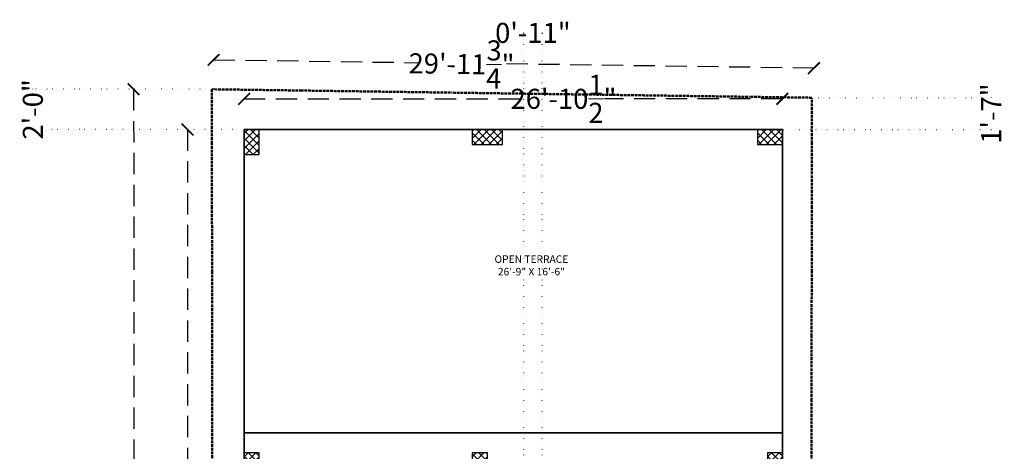
# Model space of a CAD drawing. Units: inches. Extents: x -16911 to -9621, y -48626 to -46270.
# Tile 19 of 20: x -11596 to -11006, y -46579 to -46321. Entities that reach past the tile are written whole.
import ezdxf

# ---------------------------------------------------------------- set-up
doc = ezdxf.new("R2010")
doc.units = ezdxf.units.IN
for name, pattern in [('DASHDOT', [1, 0.5, -0.25, 0, -0.25]), ('DASHED', [19.05, 12.7, -6.35]), ('DOT2', [3.175, 0, -3.175])]:
    doc.linetypes.add(name, pattern=pattern)
for name, color, linetype, lineweight in [('A-ANNO-DIMS', 2, 'Continuous', 13), ('A-AREA-IDEN', 3, 'Continuous', 18), ('A-WALL', 7, 'Continuous', 35), ('C-PROP', 6, 'DASHDOT', 50), ('column', 12, 'Continuous', 30), ('S-COLS', 1, 'Continuous', 30)]:
    doc.layers.add(name, color=color, linetype=linetype, lineweight=lineweight)
doc.styles.add('style9', font='swisscl.ttf', dxfattribs={"height": 12})
doc.dimstyles.new('Dim9', dxfattribs={"dimtxt": 10, "dimasz": 0.199219, "dimexe": 1, "dimexo": 0.5, "dimgap": 1, "dimtad": 0, "dimdec": 1, "dimzin": 0, "dimdsep": 46, "dimlunit": 4, "dimtxsty": 'style9', "dimblk": 'ARCHTICK', "dimcen": 0.09, "dimclrd": 256, "dimclrt": 256, "dimadec": 0, "dimazin": 0, "dimtfac": 1, "dimtdec": 1, "dimtix": 1, "dimtofl": 0, "dimtmove": 1, "dimatfit": 3, "dimfxl": 9, "dimtolj": 1, "dimtzin": 0, "dimlwd": -1, "dimarcsym": 0})

# ---------------------------------------------------------------- blocks, each defined once
blk = doc.blocks.new('_ArchTick')
at = {"color": 0, "linetype": 'ByBlock', "const_width": 0.15}
blk.add_lwpolyline([(-0.5, -0.5), (0.5, 0.5)], dxfattribs=at)
blk = doc.blocks.new('*D12')
at = {"layer": 'A-ANNO-DIMS', "color": 0, "linetype": 'DOT2', "lineweight": -2, "transparency": 16777216}
for p, q in [((-11479.71, -46345.34), (-11479.69, -46344.15)), ((-11120.05, -46350.39), (-11120.03, -46349.2))]:
    blk.add_line(p, q, dxfattribs=at)
at = {"layer": 'A-ANNO-DIMS', "color": 0, "linetype": 'DASHED', "lineweight": 25, "transparency": 16777216}
for p, q in [((-11479.71, -46345.15), (-11355.97, -46346.89)), ((-11120.04, -46350.2), (-11306.38, -46347.59))]:
    blk.add_line(p, q, dxfattribs=at)
at = {"layer": 'Defpoints', "color": 0, "transparency": 16777216}
for p in [(-11120.04, -46350.2), (-11479.9, -46359.07), (-11120.24, -46364.11)]:
    blk.add_point(p, dxfattribs=at)
at = {"layer": 'A-ANNO-DIMS', "color": 0, "lineweight": 25, "transparency": 16777216, "xscale": 7, "yscale": 7, "zscale": 7}
for p, rotation in [((-11479.71, -46345.15), 179.1963905603631), ((-11120.04, -46350.2), 359.196390560363)]:
    blk.add_blockref('_ArchTick', p, dxfattribs=dict(at, rotation=rotation))
at = {"layer": 'A-ANNO-DIMS', "color": 0, "transparency": 16777216, "insert": (-11331.18, -46347.68), "char_height": 12, "attachment_point": 5, "rotation": 359.19639, "style": 'style9'}
blk.add_mtext('\\A1;29\'-11{\\H1x;\\S3/4;}"', dxfattribs=at)
blk = doc.blocks.new('*D13')
at = {"layer": 'A-ANNO-DIMS', "color": 0, "linetype": 'DOT2', "lineweight": -2, "transparency": 16777216}
for p, q in [((-11527.5, -46362.82), (-11528.69, -46362.82)), ((-11527.14, -46962.82), (-11528.32, -46962.82))]:
    blk.add_line(p, q, dxfattribs=at)
at = {"layer": 'A-ANNO-DIMS', "color": 0, "linetype": 'DASHED', "lineweight": 25, "transparency": 16777216}
for p, q in [((-11527.69, -46362.82), (-11527.51, -46653.98)), ((-11527.32, -46962.82), (-11527.5, -46671.67))]:
    blk.add_line(p, q, dxfattribs=at)
at = {"layer": 'Defpoints', "color": 0, "transparency": 16777216}
for p in [(-11527.69, -46362.82), (-11508.87, -46362.81), (-11508.51, -46962.81)]:
    blk.add_point(p, dxfattribs=at)
at = {"layer": 'A-ANNO-DIMS', "color": 0, "lineweight": 25, "transparency": 16777216, "xscale": 7, "yscale": 7, "zscale": 7}
for p, rotation in [((-11527.69, -46362.82), 90.0346840750536), ((-11527.32, -46962.82), 270.0346840750536)]:
    blk.add_blockref('_ArchTick', p, dxfattribs=dict(at, rotation=rotation))
at = {"layer": 'A-ANNO-DIMS', "color": 0, "transparency": 16777216, "insert": (-11527.51, -46662.82), "char_height": 12, "attachment_point": 5, "rotation": 270.03468, "style": 'style9'}
blk.add_mtext("\\A1;50'", dxfattribs=at)
blk = doc.blocks.new('*D14')
at = {"layer": 'A-ANNO-DIMS', "color": 0, "linetype": 'DOT2', "lineweight": -2, "transparency": 16777216}
for p, q in [((-11461.47, -46368.33), (-11461.47, -46369.52)), ((-11138.92, -46368.33), (-11138.92, -46369.52))]:
    blk.add_line(p, q, dxfattribs=at)
at = {"layer": 'A-ANNO-DIMS', "color": 0, "linetype": 'DASHED', "lineweight": 25, "transparency": 16777216}
for p, q in [((-11461.47, -46368.52), (-11294.69, -46368.52)), ((-11138.92, -46368.52), (-11245.42, -46368.52))]:
    blk.add_line(p, q, dxfattribs=at)
at = {"layer": 'Defpoints', "color": 0, "transparency": 16777216}
for p in [(-11461.47, -46345.28), (-11138.92, -46345.28), (-11138.92, -46368.52)]:
    blk.add_point(p, dxfattribs=at)
at = {"layer": 'A-ANNO-DIMS', "color": 0, "lineweight": 25, "transparency": 16777216, "xscale": 7, "yscale": 7, "zscale": 7, "rotation": 180}
blk.add_blockref('_ArchTick', (-11461.47, -46368.52), dxfattribs=at)
at = {"layer": 'A-ANNO-DIMS', "color": 0, "lineweight": 25, "transparency": 16777216, "xscale": 7, "yscale": 7, "zscale": 7}
blk.add_blockref('_ArchTick', (-11138.92, -46368.52), dxfattribs=at)
at = {"layer": 'A-ANNO-DIMS', "color": 0, "transparency": 16777216, "insert": (-11270.06, -46368.52), "char_height": 12, "attachment_point": 5, "style": 'style9'}
blk.add_mtext('\\A1;26\'-10{\\H1x;\\S1/2;}"', dxfattribs=at)
blk = doc.blocks.new('*D15')
at = {"layer": 'A-ANNO-DIMS', "color": 0, "linetype": 'DOT2', "lineweight": -2, "transparency": 16777216}
for p, q in [((-11495.22, -46386.86), (-11496.4, -46386.86)), ((-11495.22, -46944.81), (-11496.4, -46944.81))]:
    blk.add_line(p, q, dxfattribs=at)
at = {"layer": 'A-ANNO-DIMS', "color": 0, "linetype": 'DASHED', "lineweight": 25, "transparency": 16777216}
for p, q in [((-11495.4, -46386.86), (-11495.4, -46648.2)), ((-11495.4, -46944.81), (-11495.4, -46683.47))]:
    blk.add_line(p, q, dxfattribs=at)
at = {"layer": 'Defpoints', "color": 0, "transparency": 16777216}
for p in [(-11461.47, -46386.86), (-11495.4, -46944.81), (-11461.47, -46944.81)]:
    blk.add_point(p, dxfattribs=at)
at = {"layer": 'A-ANNO-DIMS', "color": 0, "lineweight": 25, "transparency": 16777216, "xscale": 7, "yscale": 7, "zscale": 7}
for p, rotation in [((-11495.4, -46386.86), 90), ((-11495.4, -46944.81), 270)]:
    blk.add_blockref('_ArchTick', p, dxfattribs=dict(at, rotation=rotation))
at = {"layer": 'A-ANNO-DIMS', "color": 0, "transparency": 16777216, "insert": (-11495.4, -46665.83), "char_height": 12, "attachment_point": 5, "rotation": 90, "style": 'style9'}
blk.add_mtext('\\A1;46\'-6"', dxfattribs=at)
blk = doc.blocks.new('COLUMNS')
at = {"layer": 'column'}
h = blk.add_hatch(dxfattribs=at)
h.set_pattern_fill('ANSI37', color=256, angle=-720)
h.set_pattern_definition([(45, (21703.4588, -104481.6704), (-2.24506403, 2.24506403), []), (135, (21703.4588, -104481.6704), (-2.24506403, -2.24506403), [])])
h.paths.add_polyline_path([(-12061.47, -46401.86), (-12052.47, -46401.86), (-12052.47, -46386.86), (-12061.47, -46386.86)])
h = blk.add_hatch(dxfattribs=at)
h.set_pattern_fill('ANSI37', color=256, angle=-810)
h.set_pattern_definition([(315, (-70004.5392, -80151.7886), (2.24506403, 2.24506403), []), (45, (-70004.5392, -80151.7886), (-2.24506403, 2.24506403), [])])
h.paths.add_polyline_path([(-11924.72, -46386.86), (-11924.72, -46395.86), (-11906.72, -46395.86), (-11906.72, -46386.86)])
h = blk.add_hatch(dxfattribs=at)
h.set_pattern_fill('ANSI37', color=256, angle=-810)
h.set_pattern_definition([(315, (-69833.7395, -80151.7886), (2.24506403, 2.24506403), []), (45, (-69833.7395, -80151.7886), (-2.24506403, 2.24506403), [])])
h.paths.add_polyline_path([(-11753.92, -46386.86), (-11753.92, -46395.86), (-11738.92, -46395.86), (-11738.92, -46386.86)])
h = blk.add_hatch(dxfattribs=at)
h.set_pattern_fill('ANSI37', color=256, angle=-900)
h.set_pattern_definition([(225, (-45817.4075, 11499.4594), (2.24506403, -2.24506403), []), (315, (-45817.4075, 11499.4594), (2.24506403, 2.24506403), [])])
h.paths.add_polyline_path([(-12052.47, -46580.36), (-12061.47, -46580.36), (-12061.47, -46595.36), (-12052.47, -46595.36)])
h = blk.add_hatch(dxfattribs=at)
h.set_pattern_fill('ANSI37', color=256, angle=-720)
h.set_pattern_definition([(45, (21840.2088, -104675.1704), (-2.24506403, 2.24506403), []), (135, (21840.2088, -104675.1704), (-2.24506403, -2.24506403), [])])
h.paths.add_polyline_path([(-11924.72, -46595.36), (-11915.72, -46595.36), (-11915.72, -46580.36), (-11924.72, -46580.36)])
h = blk.add_hatch(dxfattribs=at)
h.set_pattern_fill('ANSI37', color=256, angle=-900)
h.set_pattern_definition([(225, (-45503.8578, 11499.4594), (2.24506403, -2.24506403), []), (315, (-45503.8578, 11499.4594), (2.24506403, 2.24506403), [])])
h.paths.add_polyline_path([(-11738.92, -46580.36), (-11747.92, -46580.36), (-11747.92, -46595.36), (-11738.92, -46595.36)])
h = blk.add_hatch(dxfattribs=at)
h.set_pattern_fill('ANSI37', color=256, angle=-810)
h.set_pattern_definition([(315, (-70141.2892, -80432.2886), (2.24506403, 2.24506403), []), (45, (-70141.2892, -80432.2886), (-2.24506403, 2.24506403), [])])
h.paths.add_polyline_path([(-12061.47, -46667.36), (-12061.47, -46676.36), (-12046.47, -46676.36), (-12046.47, -46667.36)])
h = blk.add_hatch(dxfattribs=at)
h.set_pattern_fill('ANSI37', color=256, angle=-810)
h.set_pattern_definition([(315, (-70010.7892, -80432.2886), (2.24506403, 2.24506403), []), (45, (-70010.7892, -80432.2886), (-2.24506403, 2.24506403), [])])
h.paths.add_polyline_path([(-11930.97, -46667.36), (-11930.97, -46676.36), (-11915.97, -46676.36), (-11915.97, -46667.36)])
h = blk.add_hatch(dxfattribs=at)
h.set_pattern_fill('ANSI37', color=256, angle=-810)
h.set_pattern_definition([(315, (-69833.7395, -80432.2886), (2.24506403, 2.24506403), []), (45, (-69833.7395, -80432.2886), (-2.24506403, 2.24506403), [])])
h.paths.add_polyline_path([(-11753.92, -46667.36), (-11753.92, -46676.36), (-11738.92, -46676.36), (-11738.92, -46667.36)])
h = blk.add_hatch(dxfattribs=at)
h.set_pattern_fill('ANSI37', color=256, angle=-540)
h.set_pattern_definition([(225, (-45817.4075, 11262.5055), (2.24506403, -2.24506403), []), (315, (-45817.4075, 11262.5055), (2.24506403, 2.24506403), [])])
h.paths.add_polyline_path([(-12052.47, -46817.31), (-12061.47, -46817.31), (-12061.47, -46832.31), (-12052.47, -46832.31)])
h = blk.add_hatch(dxfattribs=at)
h.set_pattern_fill('ANSI37', color=256, angle=-720)
h.set_pattern_definition([(45, (21885.2088, -104912.1242), (-2.24506403, 2.24506403), []), (135, (21885.2088, -104912.1242), (-2.24506403, -2.24506403), [])])
h.paths.add_polyline_path([(-11879.72, -46832.31), (-11870.72, -46832.31), (-11870.72, -46817.31), (-11879.72, -46817.31)])
h = blk.add_hatch(dxfattribs=at)
h.set_pattern_fill('ANSI37', color=256, angle=-720)
h.set_pattern_definition([(45, (22017.1023, -104912.1242), (-2.24506403, 2.24506403), []), (135, (22017.1023, -104912.1242), (-2.24506403, -2.24506403), [])])
h.paths.add_polyline_path([(-11747.83, -46832.31), (-11738.83, -46832.31), (-11738.83, -46817.31), (-11747.83, -46817.31)])
h = blk.add_hatch(dxfattribs=at)
h.set_pattern_fill('ANSI37', color=256, angle=-720)
h.set_pattern_definition([(45, (21703.4588, -105024.6242), (-2.24506403, 2.24506403), []), (135, (21703.4588, -105024.6242), (-2.24506403, -2.24506403), [])])
h.paths.add_polyline_path([(-12061.47, -46944.81), (-12052.47, -46944.81), (-12052.47, -46929.81), (-12061.47, -46929.81)])
h = blk.add_hatch(dxfattribs=at)
h.set_pattern_fill('ANSI37', color=256, angle=-810)
h.set_pattern_definition([(315, (-69959.5392, -80700.7425), (2.24506403, 2.24506403), []), (45, (-69959.5392, -80700.7425), (-2.24506403, 2.24506403), [])])
h.paths.add_polyline_path([(-11879.72, -46935.81), (-11879.72, -46944.81), (-11864.72, -46944.81), (-11864.72, -46935.81)])
h = blk.add_hatch(dxfattribs=at)
h.set_pattern_fill('ANSI37', color=256, angle=-810)
h.set_pattern_definition([(315, (-69833.7395, -80700.7425), (2.24506403, 2.24506403), []), (45, (-69833.7395, -80700.7425), (-2.24506403, 2.24506403), [])])
h.paths.add_polyline_path([(-11753.92, -46935.81), (-11753.92, -46944.81), (-11738.92, -46944.81), (-11738.92, -46935.81)])
at = {"layer": 'column', "ltscale": 0.05}
for points in [[(-12052.47, -46386.86), (-12061.47, -46386.86), (-12061.47, -46401.86), (-12052.47, -46401.86)], [(-11906.72, -46395.86), (-11906.72, -46386.86), (-11924.72, -46386.86), (-11924.72, -46395.86)], [(-11738.92, -46395.86), (-11738.92, -46386.86), (-11753.92, -46386.86), (-11753.92, -46395.86)], [(-12061.47, -46595.36), (-12052.47, -46595.36), (-12052.47, -46580.36), (-12061.47, -46580.36)], [(-11915.72, -46580.36), (-11924.72, -46580.36), (-11924.72, -46595.36), (-11915.72, -46595.36)], [(-11747.92, -46595.36), (-11738.92, -46595.36), (-11738.92, -46580.36), (-11747.92, -46580.36)], [(-12046.47, -46676.36), (-12046.47, -46667.36), (-12061.47, -46667.36), (-12061.47, -46676.36)], [(-11915.97, -46676.36), (-11915.97, -46667.36), (-11930.97, -46667.36), (-11930.97, -46676.36)], [(-11738.92, -46676.36), (-11738.92, -46667.36), (-11753.92, -46667.36), (-11753.92, -46676.36)], [(-12061.47, -46832.31), (-12052.47, -46832.31), (-12052.47, -46817.31), (-12061.47, -46817.31)], [(-11870.72, -46817.31), (-11879.72, -46817.31), (-11879.72, -46832.31), (-11870.72, -46832.31)], [(-11738.83, -46817.31), (-11747.83, -46817.31), (-11747.83, -46832.31), (-11738.83, -46832.31)], [(-12052.47, -46929.81), (-12061.47, -46929.81), (-12061.47, -46944.81), (-12052.47, -46944.81)], [(-11864.72, -46944.81), (-11864.72, -46935.81), (-11879.72, -46935.81), (-11879.72, -46944.81)], [(-11738.92, -46944.81), (-11738.92, -46935.81), (-11753.92, -46935.81), (-11753.92, -46944.81)]]:
    blk.add_lwpolyline(points, close=True, dxfattribs=at)
blk = doc.blocks.new('*D123')
at = {"layer": 'A-ANNO-DIMS', "linetype": 'DASHED', "transparency": 16777216}
for p, q in [((-11293.92, -46329.06), (-11294.12, -46329.06)), ((-11282.92, -46329.06), (-11282.73, -46329.06))]:
    blk.add_line(p, q, dxfattribs=at)
at = {"layer": 'A-ANNO-DIMS', "color": 0, "linetype": 'DOT2', "lineweight": -2, "transparency": 16777216}
for p, q in [((-11293.92, -46594.86), (-11293.92, -46328.06)), ((-11282.92, -46594.86), (-11282.92, -46328.06))]:
    blk.add_line(p, q, dxfattribs=at)
at = {"layer": 'Defpoints', "color": 0, "transparency": 16777216}
for p in [(-11282.92, -46329.06), (-11293.92, -46595.36), (-11282.92, -46595.36)]:
    blk.add_point(p, dxfattribs=at)
at = {"layer": 'A-ANNO-DIMS', "transparency": 16777216, "xscale": 0.19921875, "yscale": 0.19921875, "zscale": 0.19921875}
blk.add_blockref('_ArchTick', (-11293.92, -46329.06), dxfattribs=at)
at = {"layer": 'A-ANNO-DIMS', "transparency": 16777216, "xscale": 0.19921875, "yscale": 0.19921875, "zscale": 0.19921875, "rotation": 180}
blk.add_blockref('_ArchTick', (-11282.92, -46329.06), dxfattribs=at)
at = {"layer": 'A-ANNO-DIMS', "transparency": 16777216, "insert": (-11288.42, -46329.06), "char_height": 12, "attachment_point": 5, "style": 'style9'}
blk.add_mtext('\\A1;0\'-11"', dxfattribs=at)
blk = doc.blocks.new('*D126')
at = {"layer": 'A-ANNO-DIMS', "color": 0, "linetype": 'DOT2', "lineweight": -2, "transparency": 16777216}
for p, q in [((-11481.34, -46362.81), (-11589.1, -46362.81)), ((-11461.97, -46386.86), (-11589.1, -46386.86))]:
    blk.add_line(p, q, dxfattribs=at)
at = {"layer": 'A-ANNO-DIMS', "linetype": 'DASHED', "transparency": 16777216}
for p, q in [((-11588.1, -46362.81), (-11588.1, -46362.61)), ((-11588.1, -46386.86), (-11588.1, -46387.05))]:
    blk.add_line(p, q, dxfattribs=at)
at = {"layer": 'Defpoints', "color": 0, "transparency": 16777216}
for p in [(-11480.84, -46362.81), (-11588.1, -46386.86), (-11461.47, -46386.86)]:
    blk.add_point(p, dxfattribs=at)
at = {"layer": 'A-ANNO-DIMS', "transparency": 16777216, "xscale": 0.19921875, "yscale": 0.19921875, "zscale": 0.19921875}
for p, rotation in [((-11588.1, -46362.81), 270), ((-11588.1, -46386.86), 90)]:
    blk.add_blockref('_ArchTick', p, dxfattribs=dict(at, rotation=rotation))
at = {"layer": 'A-ANNO-DIMS', "transparency": 16777216, "insert": (-11588.1, -46374.83), "char_height": 12, "attachment_point": 5, "rotation": 90, "style": 'style9'}
blk.add_mtext('\\A1;2\'-0"', dxfattribs=at)
blk = doc.blocks.new('*D127')
at = {"layer": 'A-ANNO-DIMS', "color": 0, "linetype": 'DOT2', "lineweight": -2, "transparency": 16777216}
for p, q in [((-11120.67, -46367.86), (-11012.8, -46367.86)), ((-11138.42, -46386.86), (-11012.8, -46386.86))]:
    blk.add_line(p, q, dxfattribs=at)
at = {"layer": 'A-ANNO-DIMS', "linetype": 'DASHED', "transparency": 16777216}
for p, q in [((-11013.8, -46367.86), (-11013.8, -46367.66)), ((-11013.8, -46386.86), (-11013.8, -46387.05))]:
    blk.add_line(p, q, dxfattribs=at)
at = {"layer": 'Defpoints', "color": 0, "transparency": 16777216}
for p in [(-11121.17, -46367.86), (-11138.92, -46386.86), (-11013.8, -46386.86)]:
    blk.add_point(p, dxfattribs=at)
at = {"layer": 'A-ANNO-DIMS', "transparency": 16777216, "xscale": 0.19921875, "yscale": 0.19921875, "zscale": 0.19921875}
for p, rotation in [((-11013.8, -46367.86), 270), ((-11013.8, -46386.86), 90)]:
    blk.add_blockref('_ArchTick', p, dxfattribs=dict(at, rotation=rotation))
at = {"layer": 'A-ANNO-DIMS', "transparency": 16777216, "insert": (-11013.8, -46377.36), "char_height": 12, "attachment_point": 5, "rotation": 90, "style": 'style9'}
blk.add_mtext('\\A1;1\'-7"', dxfattribs=at)

msp = doc.modelspace()

# ---------------------------------------------------------------- linework, layer by layer
at = {"layer": 'A-WALL'}
for p, q in [((-11138.925, -46386.855), (-11461.474, -46386.855)), ((-11461.474, -46586.355), (-11461.474, -46386.855)), ((-11138.925, -46386.855), (-11138.925, -46586.355)), ((-11461.474, -46568.355), (-11138.925, -46568.355))]:
    msp.add_line(p, q, dxfattribs=at)
at = {"layer": 'C-PROP'}
msp.add_lwpolyline([(-11480.474, -46962.809), (-11120.293, -46969.035), (-11119.732, -46940.446), (-11120.395, -46855.606), (-11121.561, -46609.511), (-11121.175, -46367.855), (-11480.838, -46362.811), (-11480.3, -46762.955)], close=True, dxfattribs=at)

# ---------------------------------------------------------------- block references
at = {"layer": 'S-COLS'}
msp.add_blockref('COLUMNS', (600, 0), dxfattribs=at)

# ---------------------------------------------------------------- texts
at = {"layer": 'A-AREA-IDEN', "ltscale": 10, "insert": (-11319.218, -46462.207), "char_height": 4.5, "width": 59.80751, "attachment_point": 1, "style": 'style9'}
msp.add_mtext('\\A1;\\pxqc;{\\fCentury Gothic|b0|i0|c0|p34;OPEN TERRACE\\P26\'-9" X 16\'-6"}', dxfattribs=at)

# ---------------------------------------------------------------- dimensions: what is measured, and where the dimension line sits
at = {"layer": 'A-ANNO-DIMS'}
dim = msp.add_linear_dim(base=(-11282.925, -46329.061), p1=(-11293.925, -46595.355), p2=(-11282.925, -46595.355), dimstyle='Dim9', override={"dimdec": 1, "dimlfac": 1, "dimrnd": 0, "dimzin": 1, "dimdsep": 46, "dimlunit": 4, "dimfrac": 2}, dxfattribs=at)
dim.commit()
dim.dimension.update_dxf_attribs({"geometry": '*D123', "text_midpoint": (-11288.425, -46329.061)})
dim = msp.add_linear_dim(base=(-11120.044, -46350.199), p1=(-11479.902, -46359.069), p2=(-11120.239, -46364.114), angle=359.196391, dimstyle='Dim9', override={"dimtxt": 12, "dimasz": 7, "dimdec": 2, "dimclrd": 0, "dimclre": 0, "dimclrt": 0, "dimtdec": 2, "dimfxl": 0.1875, "dimfxlon": 1, "dimlwd": 25, "dimarcsym": 2}, dxfattribs=at)
dim.commit()
dim.dimension.update_dxf_attribs({"geometry": '*D12', "text_midpoint": (-11331.179, -46347.677), "dimtype": 161})
dim = msp.add_linear_dim(base=(-11138.925, -46368.516), p1=(-11461.474, -46345.28), p2=(-11138.925, -46345.28), dimstyle='Dim9', override={"dimtxt": 12, "dimasz": 7, "dimdec": 2, "dimclrd": 0, "dimclre": 0, "dimclrt": 0, "dimtdec": 2, "dimfxl": 0.1875, "dimfxlon": 1, "dimlwd": 25, "dimarcsym": 2}, dxfattribs=at)
dim.commit()
dim.dimension.update_dxf_attribs({"geometry": '*D14', "text_midpoint": (-11270.059, -46368.516), "dimtype": 160})
for base, p1, p2, override, picture, middle in [((-11588.099, -46386.855), (-11480.838, -46362.811), (-11461.474, -46386.855), {"dimdec": 1, "dimlfac": 1, "dimrnd": 0, "dimzin": 1, "dimdsep": 46, "dimlunit": 4, "dimfrac": 2}, '*D126', (-11588.099, -46374.833)), ((-11013.797, -46386.855), (-11121.175, -46367.855), (-11138.925, -46386.855), {"dimdec": 1, "dimlfac": 1, "dimrnd": 0, "dimzin": 1, "dimdsep": 46, "dimlunit": 4, "dimfrac": 2}, '*D127', (-11013.797, -46377.355)), ((-11495.403, -46944.809), (-11461.474, -46386.855), (-11461.474, -46944.809), {"dimtxt": 12, "dimasz": 7, "dimdec": 2, "dimclrd": 0, "dimclre": 0, "dimclrt": 0, "dimtdec": 2, "dimfxl": 0.1875, "dimfxlon": 1, "dimlwd": 25, "dimarcsym": 2}, '*D15', (-11495.403, -46665.832))]:
    dim = msp.add_linear_dim(base=base, p1=p1, p2=p2, angle=90, dimstyle='Dim9', override=override, dxfattribs=at)
    dim.commit()
    dim.dimension.update_dxf_attribs({"geometry": picture, "text_midpoint": middle})
dim = msp.add_aligned_dim(p1=(-11508.507, -46962.809), p2=(-11508.87, -46362.811), distance=18.817, dimstyle='Dim9', override={"dimtxt": 12, "dimasz": 7, "dimdec": 2, "dimclrd": 0, "dimclre": 0, "dimclrt": 0, "dimtdec": 2, "dimfxl": 0.1875, "dimfxlon": 1, "dimlwd": 25, "dimarcsym": 2}, dxfattribs=at)
dim.commit()
dim.dimension.update_dxf_attribs({"geometry": '*D13', "text_midpoint": (-11527.505, -46662.821)})

doc.saveas('drawing.dxf')
